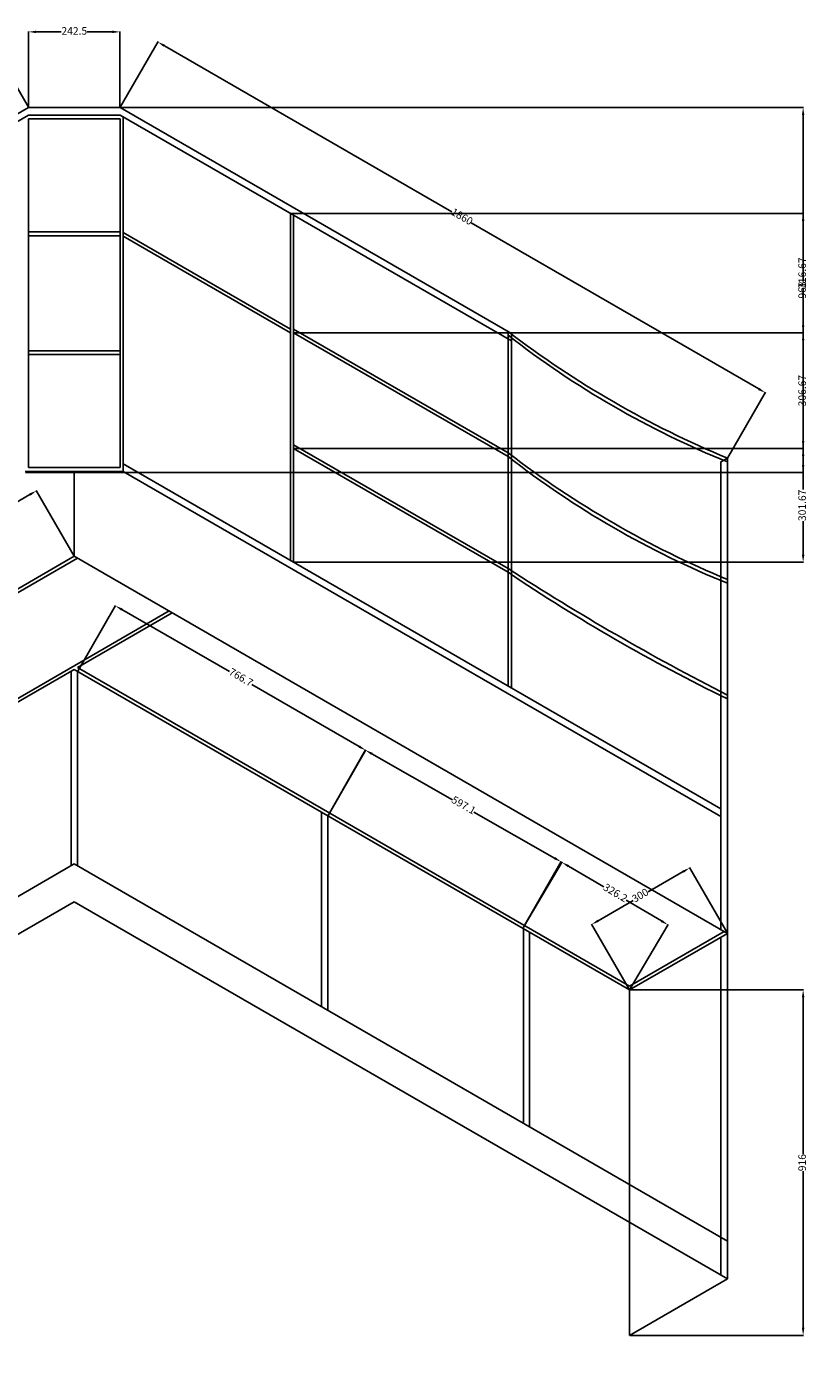
# Model space of a CAD drawing. Units: millimetres. Extents: x 78378 to 86415, y 148682 to 152721.
# Tile 18 of 18: x 84344 to 86415, y 149152 to 152721. Entities that reach past the tile are written whole.
import ezdxf

# ---------------------------------------------------------------- set-up
doc = ezdxf.new("R2010")
doc.units = ezdxf.units.MM
for name, color, linetype, lineweight in [('A-ANNO-DIMS', 2, 'Continuous', 18), ('A-ANNO-NPLT', 8, 'Continuous', 13), ('A-FURN', 4, 'Continuous', 25)]:
    doc.layers.add(name, color=color, linetype=linetype, lineweight=lineweight)
doc.styles.get("Standard").update_dxf_attribs({"font": 'arial.ttf'})
doc.dimstyles.new('ISO-25', dxfattribs={"dimtxt": 20, "dimasz": 20, "dimexe": 1.25, "dimexo": 0.625, "dimtad": 0, "dimdec": 1, "dimtxsty": 'Standard', "dimcen": 2.5, "dimadec": 0, "dimazin": 0, "dimtfac": 1, "dimtdec": 1, "dimtmove": 0, "dimatfit": 3, "dimfxl": 1, "dimarcsym": 0})

# ---------------------------------------------------------------- blocks, each defined once
blk = doc.blocks.new('*D35')
at = {"layer": 'A-ANNO-DIMS', "color": 0, "lineweight": -2, "transparency": 16777216}
for p, q in [((84347.7, 152508.2), (84247.2, 152682.4)), ((84230.5, 152671.3), (83252.4, 152106.6)), ((82221.3, 151511.3), (83199.4, 152076)), ((82303.9, 151328.2), (82203.4, 151502.4))]:
    blk.add_line(p, q, dxfattribs=at)
at = {"layer": 'A-ANNO-DIMS', "color": 0, "transparency": 16777216}
for points in [[(84228.8, 152674.2), (84232.2, 152668.4), (84247.8, 152681.3)], [(82219.6, 151514.2), (82223, 151508.4), (82204, 151501.3)]]:
    blk.add_solid(points, dxfattribs=at)
at = {"layer": 'Defpoints', "color": 0, "transparency": 16777216}
for p in [(84247.8, 152681.3), (84348.1, 152507.7), (82304.2, 151327.7)]:
    blk.add_point(p, dxfattribs=at)
at = {"layer": 'A-ANNO-DIMS', "color": 0, "transparency": 16777216, "insert": (83225.9, 152091.3), "char_height": 20, "attachment_point": 5, "rotation": 30}
blk.add_mtext('2360', dxfattribs=at)
blk = doc.blocks.new('*D36')
at = {"layer": 'A-ANNO-DIMS', "color": 0, "lineweight": -2, "transparency": 16777216}
for p, q in [((84590.9, 152508.2), (84691.4, 152682.4)), ((84708.1, 152671.3), (85470.6, 152231.1)), ((86284.3, 151761.3), (85521.8, 152201.6)), ((86201.7, 151578.2), (86302.2, 151752.4))]:
    blk.add_line(p, q, dxfattribs=at)
at = {"layer": 'A-ANNO-DIMS', "color": 0, "transparency": 16777216}
for points in [[(84709.8, 152674.2), (84706.5, 152668.4), (84690.8, 152681.3)], [(86286, 151764.2), (86282.6, 151758.4), (86301.6, 151751.3)]]:
    blk.add_solid(points, dxfattribs=at)
at = {"layer": 'Defpoints', "color": 0, "transparency": 16777216}
for p in [(84590.5, 152507.7), (86301.6, 151751.3), (86201.4, 151577.7)]:
    blk.add_point(p, dxfattribs=at)
at = {"layer": 'A-ANNO-DIMS', "color": 0, "transparency": 16777216, "insert": (85496.2, 152216.3), "char_height": 20, "attachment_point": 5, "rotation": 330}
blk.add_mtext('1860', dxfattribs=at)
blk = doc.blocks.new('*D37')
at = {"layer": 'A-ANNO-DIMS', "color": 0, "lineweight": -2, "transparency": 16777216}
for p, q in [((84348.1, 152508.3), (84348.1, 152709.4)), ((84590.5, 152508.3), (84590.5, 152709.4)), ((84368.1, 152708.2), (84434.7, 152708.2)), ((84570.5, 152708.2), (84503.9, 152708.2))]:
    blk.add_line(p, q, dxfattribs=at)
at = {"layer": 'A-ANNO-DIMS', "color": 0, "transparency": 16777216}
for points in [[(84368.1, 152711.5), (84368.1, 152704.9), (84348.1, 152708.2)], [(84570.5, 152711.5), (84570.5, 152704.9), (84590.5, 152708.2)]]:
    blk.add_solid(points, dxfattribs=at)
at = {"layer": 'Defpoints', "color": 0, "transparency": 16777216}
for p in [(84590.5, 152708.2), (84348.1, 152507.7), (84590.5, 152507.7)]:
    blk.add_point(p, dxfattribs=at)
at = {"layer": 'A-ANNO-DIMS', "color": 0, "transparency": 16777216, "insert": (84469.3, 152708.2), "char_height": 20, "attachment_point": 5}
blk.add_mtext('242.5', dxfattribs=at)
blk = doc.blocks.new('*D38')
at = {"layer": 'A-ANNO-DIMS', "color": 0, "lineweight": -2, "transparency": 16777216}
for p, q in [((84348.7, 152507.7), (86403.1, 152507.7)), ((86401.9, 152487.7), (86401.9, 152046.5)), ((86401.9, 151559.8), (86401.9, 152001)), ((84340, 151539.8), (86403.1, 151539.8))]:
    blk.add_line(p, q, dxfattribs=at)
at = {"layer": 'A-ANNO-DIMS', "color": 0, "transparency": 16777216}
for points in [[(86398.5, 152487.7), (86405.2, 152487.7), (86401.9, 152507.7)], [(86398.5, 151559.8), (86405.2, 151559.8), (86401.9, 151539.8)]]:
    blk.add_solid(points, dxfattribs=at)
at = {"layer": 'Defpoints', "color": 0, "transparency": 16777216}
for p in [(84348.1, 152507.7), (86401.9, 152507.7), (84339.4, 151539.8)]:
    blk.add_point(p, dxfattribs=at)
at = {"layer": 'A-ANNO-DIMS', "color": 0, "transparency": 16777216, "insert": (86401.9, 152023.7), "char_height": 20, "attachment_point": 5, "rotation": 90}
blk.add_mtext('968', dxfattribs=at)
blk = doc.blocks.new('*D41')
at = {"layer": 'A-ANNO-DIMS', "color": 0, "lineweight": -2, "transparency": 16777216}
for p, q in [((84351.7, 151481.3), (83937.7, 151242.3)), ((84469, 151318.2), (84368.4, 151492.4)), ((83452.3, 150962), (83866.3, 151201.1)), ((83534.9, 150778.9), (83434.4, 150953.1))]:
    blk.add_line(p, q, dxfattribs=at)
at = {"layer": 'A-ANNO-DIMS', "color": 0, "transparency": 16777216}
for points in [[(84350.1, 151484.2), (84353.4, 151478.4), (84369.1, 151491.3)], [(83450.6, 150964.9), (83454, 150959.2), (83435, 150952)]]:
    blk.add_solid(points, dxfattribs=at)
at = {"layer": 'Defpoints', "color": 0, "transparency": 16777216}
for p in [(84369.1, 151491.3), (84469.3, 151317.7), (83535.2, 150778.4)]:
    blk.add_point(p, dxfattribs=at)
at = {"layer": 'A-ANNO-DIMS', "color": 0, "transparency": 16777216, "insert": (83902, 151221.7), "char_height": 20, "attachment_point": 5, "rotation": 30}
blk.add_mtext('1078.6', dxfattribs=at)
blk = doc.blocks.new('*D46')
at = {"layer": 'A-ANNO-DIMS', "color": 0, "lineweight": -2, "transparency": 16777216}
for p, q in [((85942.2, 150167.7), (86403.1, 150167.7)), ((86401.9, 150147.7), (86401.9, 149732.4)), ((86401.9, 149271.7), (86401.9, 149687)), ((85942.2, 149251.7), (86403.1, 149251.7))]:
    blk.add_line(p, q, dxfattribs=at)
at = {"layer": 'A-ANNO-DIMS', "color": 0, "transparency": 16777216}
for points in [[(86398.5, 150147.7), (86405.2, 150147.7), (86401.9, 150167.7)], [(86398.5, 149271.7), (86405.2, 149271.7), (86401.9, 149251.7)]]:
    blk.add_solid(points, dxfattribs=at)
at = {"layer": 'Defpoints', "color": 0, "transparency": 16777216}
for p in [(85941.5, 150167.7), (86401.9, 150167.7), (85941.5, 149251.7)]:
    blk.add_point(p, dxfattribs=at)
at = {"layer": 'A-ANNO-DIMS', "color": 0, "transparency": 16777216, "insert": (86401.9, 149709.7), "char_height": 20, "attachment_point": 5, "rotation": 90}
blk.add_mtext('916', dxfattribs=at)
blk = doc.blocks.new('*D47')
at = {"layer": 'A-ANNO-DIMS', "color": 0, "lineweight": -2, "transparency": 16777216}
for p, q in [((84478.3, 151013.2), (84578.8, 151187.4)), ((84595.5, 151176.3), (84880.5, 151011.8)), ((85224.8, 150813), (84939.9, 150977.5)), ((85142.2, 150629.9), (85242.8, 150804.1))]:
    blk.add_line(p, q, dxfattribs=at)
at = {"layer": 'A-ANNO-DIMS', "color": 0, "transparency": 16777216}
for points in [[(84597.2, 151179.2), (84593.9, 151173.4), (84578.2, 151186.3)], [(85226.5, 150815.9), (85223.2, 150810.1), (85242.2, 150803)]]:
    blk.add_solid(points, dxfattribs=at)
at = {"layer": 'Defpoints', "color": 0, "transparency": 16777216}
for p in [(84478, 151012.7), (85242.2, 150803), (85141.9, 150629.4)]:
    blk.add_point(p, dxfattribs=at)
at = {"layer": 'A-ANNO-DIMS', "color": 0, "transparency": 16777216, "insert": (84910.2, 150994.7), "char_height": 20, "attachment_point": 5, "rotation": 330}
blk.add_mtext('766.7', dxfattribs=at)
blk = doc.blocks.new('*D48')
at = {"layer": 'A-ANNO-DIMS', "color": 0, "lineweight": -2, "transparency": 16777216}
for p, q in [((85142.2, 150629.9), (85241.9, 150804.6)), ((85258.7, 150793.6), (85472.4, 150671.6)), ((85742.5, 150517.4), (85528.8, 150639.4)), ((85660.8, 150333.9), (85760.5, 150508.6))]:
    blk.add_line(p, q, dxfattribs=at)
at = {"layer": 'A-ANNO-DIMS', "color": 0, "transparency": 16777216}
for points in [[(85260.3, 150796.5), (85257, 150790.7), (85241.3, 150803.5)], [(85744.2, 150520.3), (85740.9, 150514.5), (85759.9, 150507.5)]]:
    blk.add_solid(points, dxfattribs=at)
at = {"layer": 'Defpoints', "color": 0, "transparency": 16777216}
for p in [(85141.9, 150629.4), (85759.9, 150507.5), (85660.5, 150333.4)]:
    blk.add_point(p, dxfattribs=at)
at = {"layer": 'A-ANNO-DIMS', "color": 0, "transparency": 16777216, "insert": (85500.6, 150655.5), "char_height": 20, "attachment_point": 5, "rotation": 330.2843}
blk.add_mtext('597.1', dxfattribs=at)
blk = doc.blocks.new('*D49')
at = {"layer": 'A-ANNO-DIMS', "color": 0, "lineweight": -2, "transparency": 16777216}
for p, q in [((85660.8, 150333.9), (85763, 150507.2)), ((85779.6, 150495.9), (85873.3, 150440.7)), ((86026.1, 150350.6), (85932.4, 150405.9)), ((85941.9, 150168.2), (86044, 150341.5))]:
    blk.add_line(p, q, dxfattribs=at)
at = {"layer": 'A-ANNO-DIMS', "color": 0, "transparency": 16777216}
for points in [[(85781.3, 150498.8), (85777.9, 150493.1), (85762.3, 150506.1)], [(86027.8, 150353.4), (86024.5, 150347.7), (86043.4, 150340.4)]]:
    blk.add_solid(points, dxfattribs=at)
at = {"layer": 'Defpoints', "color": 0, "transparency": 16777216}
for p in [(85660.5, 150333.4), (86043.4, 150340.4), (85941.5, 150167.7)]:
    blk.add_point(p, dxfattribs=at)
at = {"layer": 'A-ANNO-DIMS', "color": 0, "transparency": 16777216, "insert": (85902.9, 150423.3), "char_height": 20, "attachment_point": 5, "rotation": 329.4797}
blk.add_mtext('326.2', dxfattribs=at)
blk = doc.blocks.new('*D50')
at = {"layer": 'A-ANNO-DIMS', "color": 0, "lineweight": -2, "transparency": 16777216}
for p, q in [((86083.8, 150481.3), (85990.8, 150427.7)), ((86201, 150318.2), (86100.5, 150492.4)), ((85858.6, 150351.3), (85951.6, 150405)), ((85941.2, 150168.2), (85840.7, 150342.4))]:
    blk.add_line(p, q, dxfattribs=at)
at = {"layer": 'A-ANNO-DIMS', "color": 0, "transparency": 16777216}
for points in [[(86082.1, 150484.2), (86085.5, 150478.4), (86101.1, 150491.3)], [(85857, 150354.2), (85860.3, 150348.4), (85841.3, 150341.3)]]:
    blk.add_solid(points, dxfattribs=at)
at = {"layer": 'Defpoints', "color": 0, "transparency": 16777216}
for p in [(86101.1, 150491.3), (86201.4, 150317.7), (85941.5, 150167.7)]:
    blk.add_point(p, dxfattribs=at)
at = {"layer": 'A-ANNO-DIMS', "color": 0, "transparency": 16777216, "insert": (85971.2, 150416.3), "char_height": 20, "attachment_point": 5, "rotation": 30}
blk.add_mtext('300', dxfattribs=at)
blk = doc.blocks.new('*D51')
at = {"layer": 'A-ANNO-DIMS', "color": 0, "lineweight": -2, "transparency": 16777216}
for p, q in [((85051.6, 151603.5), (86403.1, 151603.5)), ((86401.9, 151583.5), (86401.9, 151494.8)), ((86401.9, 151321.9), (86401.9, 151410.6)), ((85051.6, 151301.9), (86403.1, 151301.9))]:
    blk.add_line(p, q, dxfattribs=at)
at = {"layer": 'A-ANNO-DIMS', "color": 0, "transparency": 16777216}
for points in [[(86398.5, 151583.5), (86405.2, 151583.5), (86401.9, 151603.5)], [(86398.5, 151321.9), (86405.2, 151321.9), (86401.9, 151301.9)]]:
    blk.add_solid(points, dxfattribs=at)
at = {"layer": 'Defpoints', "color": 0, "transparency": 16777216}
for p in [(85051, 151603.5), (86401.9, 151603.5), (85051, 151301.9)]:
    blk.add_point(p, dxfattribs=at)
at = {"layer": 'A-ANNO-DIMS', "color": 0, "transparency": 16777216, "insert": (86401.9, 151452.7), "char_height": 20, "attachment_point": 5, "rotation": 90}
blk.add_mtext('301.67', dxfattribs=at)
blk = doc.blocks.new('*D52')
at = {"layer": 'A-ANNO-DIMS', "color": 0, "lineweight": -2, "transparency": 16777216}
for p, q in [((85051.6, 151910.2), (86403.1, 151910.2)), ((86401.9, 151890.2), (86401.9, 151799)), ((86401.9, 151623.5), (86401.9, 151714.7)), ((85051.6, 151603.5), (86403.1, 151603.5))]:
    blk.add_line(p, q, dxfattribs=at)
at = {"layer": 'A-ANNO-DIMS', "color": 0, "transparency": 16777216}
for points in [[(86398.5, 151890.2), (86405.2, 151890.2), (86401.9, 151910.2)], [(86398.5, 151623.5), (86405.2, 151623.5), (86401.9, 151603.5)]]:
    blk.add_solid(points, dxfattribs=at)
at = {"layer": 'Defpoints', "color": 0, "transparency": 16777216}
for p in [(85051, 151910.2), (86401.9, 151910.2), (85051, 151603.5)]:
    blk.add_point(p, dxfattribs=at)
at = {"layer": 'A-ANNO-DIMS', "color": 0, "transparency": 16777216, "insert": (86401.9, 151756.9), "char_height": 20, "attachment_point": 5, "rotation": 90}
blk.add_mtext('306.67', dxfattribs=at)
blk = doc.blocks.new('*D53')
at = {"layer": 'A-ANNO-DIMS', "color": 0, "lineweight": -2, "transparency": 16777216}
for p, q in [((85043, 152226.9), (86403.1, 152226.9)), ((86401.9, 152206.9), (86401.9, 152110.7)), ((86401.9, 151930.2), (86401.9, 152026.4)), ((85051.6, 151910.2), (86403.1, 151910.2))]:
    blk.add_line(p, q, dxfattribs=at)
at = {"layer": 'A-ANNO-DIMS', "color": 0, "transparency": 16777216}
for points in [[(86398.5, 152206.9), (86405.2, 152206.9), (86401.9, 152226.9)], [(86398.5, 151930.2), (86405.2, 151930.2), (86401.9, 151910.2)]]:
    blk.add_solid(points, dxfattribs=at)
at = {"layer": 'Defpoints', "color": 0, "transparency": 16777216}
for p in [(85042.3, 152226.9), (86401.9, 152226.9), (85051, 151910.2)]:
    blk.add_point(p, dxfattribs=at)
at = {"layer": 'A-ANNO-DIMS', "color": 0, "transparency": 16777216, "insert": (86401.9, 152068.5), "char_height": 20, "attachment_point": 5, "rotation": 90}
blk.add_mtext('316.67', dxfattribs=at)

msp = doc.modelspace()

# ---------------------------------------------------------------- linework, layer by layer
at = {"layer": 'A-ANNO-NPLT'}
for p in [(85046.6562, 152224.3613), (84348.0623, 152172.6946), (84590.5495, 152172.6946), (85050.9863, 151915.1946), (84348.0623, 151857.6946), (84590.5495, 151857.6946), (85050.9863, 151608.528), (85628.3366, 151581.8613), (85628.3366, 151275.1946)]:
    msp.add_point(p, dxfattribs=at)
at = {"layer": 'A-FURN'}
for p, q in [((82304.2424, 151327.6946), (84348.0623, 152507.6946)), ((84590.5495, 152507.6946), (84348.0623, 152507.6946)), ((84590.5495, 152507.6946), (85628.3366, 151908.528)), ((83953.1548, 152259.6946), (84348.0623, 152487.6946)), ((84348.0623, 152487.6946), (84590.5495, 152487.6946)), ((84348.0623, 152477.6946), (84348.0623, 151552.6946)), ((84348.0623, 152477.6946), (84590.5495, 152477.6946)), ((84590.5495, 152487.6946), (85628.3366, 151888.528)), ((84590.5495, 152477.6946), (84590.5495, 151552.6946)), ((84599.2097, 152482.6946), (84599.2097, 151542.6946)), ((85042.326, 152226.8613), (85042.326, 151306.8613)), ((85050.9863, 152221.8613), (85050.9863, 151301.8613)), ((84590.5495, 152177.6946), (84348.0623, 152177.6946)), ((85042.326, 151920.1946), (84599.2097, 152176.028)), ((84590.5495, 152167.6946), (84348.0623, 152167.6946)), ((85042.326, 151910.1946), (84599.2097, 152166.028)), ((85050.9863, 151920.1946), (85619.6763, 151591.8613)), ((85050.9863, 151910.1946), (85619.6763, 151581.8613)), ((85619.6763, 151913.528), (85619.6763, 150973.528)), ((85628.3366, 151908.528), (85628.3366, 150968.528)), ((84348.0623, 151862.6946), (84590.5495, 151862.6946)), ((84348.0623, 151852.6946), (84590.5495, 151852.6946)), ((85050.9863, 151613.528), (85619.6763, 151285.1946)), ((85050.9863, 151603.528), (85619.6763, 151275.1946)), ((86184.0362, 151567.6946), (86201.3567, 151577.6946)), ((86184.0362, 151567.6946), (86184.0362, 150327.6946)), ((86201.3567, 151577.6946), (86201.3567, 149401.6946)), ((84599.2097, 151542.6946), (84339.4021, 151542.6946)), ((84590.5495, 151552.6946), (84348.0623, 151552.6946)), ((84469.3059, 151542.6946), (84469.3059, 151317.6946)), ((84469.3059, 151542.6946), (84469.3059, 151317.6946)), ((84599.2097, 151562.6946), (86184.0362, 150647.6946)), ((84599.2097, 151542.6946), (86184.0362, 150627.6946)), ((84469.3059, 151317.6946), (83535.2323, 150778.407)), ((84469.3059, 151317.6946), (86201.3567, 150317.6946)), ((84477.9662, 151312.6946), (83535.2323, 150768.407)), ((84720.4533, 151172.6946), (83535.2323, 150488.407)), ((84477.9662, 151022.6946), (84729.1135, 151167.6946)), ((84469.3059, 151017.6946), (83535.2323, 150478.407)), ((84460.6456, 151012.6946), (84460.6456, 150496.6946)), ((84460.6456, 151012.6946), (84460.6456, 150496.6946)), ((84469.3059, 151017.6946), (85941.5491, 150167.6946)), ((84477.9662, 151022.6946), (85941.5491, 150177.6946)), ((84477.9662, 151012.6946), (84477.9662, 150496.6946)), ((84477.9662, 151012.6946), (84477.9662, 150496.6946)), ((85124.5985, 150639.3613), (85124.5985, 150123.3613)), ((85141.919, 150629.3613), (85141.919, 150113.3613)), ((83543.8926, 149967.407), (84469.3059, 150501.6946)), ((84469.3059, 150501.6946), (86201.3567, 149501.6946)), ((82304.2424, 149151.6946), (84469.3059, 150401.6946)), ((84469.3059, 150401.6946), (86201.3567, 149401.6946)), ((85660.5176, 150333.3692), (85660.5176, 149817.3692)), ((85675.968, 150321.028), (85675.968, 149805.028)), ((85941.5491, 150177.6946), (86192.6965, 150322.6946)), ((85941.5491, 150167.6946), (86201.3567, 150317.6946)), ((86184.0362, 150307.6946), (86184.0362, 149411.6946)), ((85941.5491, 149251.6946), (85941.5491, 150167.6946)), ((86201.3567, 149401.6946), (85941.5491, 149251.6946))]:
    msp.add_line(p, q, dxfattribs=at)
for centre, radius, start, end in [((87200.6508, 153980.1894), 2602.0318, 232.5843878, 247.4156122), ((87119.6642, 153829.9165), 2441.5029, 232.0937908, 247.9062092), ((87200.6508, 153658.5227), 2602.0318, 232.5843878, 247.4156122), ((87119.6642, 153508.2499), 2441.5029, 232.0937908, 247.9062092), ((89190.7083, 156798.8207), 6569.1184, 237.07034061, 242.92965939), ((88284.6881, 155219.4638), 4760.2045, 235.954411, 244.045589)]:
    msp.add_arc(centre, radius, start, end, dxfattribs=at)

# ---------------------------------------------------------------- dimensions: what is measured, and where the dimension line sits
at = {"layer": 'A-ANNO-DIMS'}
dim = msp.add_linear_dim(base=(84590.5495, 152708.1946), p1=(84348.0623, 152507.6946), p2=(84590.5495, 152507.6946), dimstyle='ISO-25', override={"dimdec": 1, "dimlfac": 1, "dimrnd": 0, "dimzin": 0, "dimdsep": 46, "dimlunit": 2}, dxfattribs=at)
dim.commit()
dim.dimension.update_dxf_attribs({"geometry": '*D37', "text_midpoint": (84469.3059, 152708.1946)})
for base, p1, p2, angle, override, picture, middle in [((84247.8123, 152681.3327), (82304.2424, 151327.6946), (84348.0623, 152507.6946), 30, {"dimdec": 0, "dimlfac": 1, "dimrnd": 0, "dimzin": 0, "dimdsep": 46, "dimlunit": 2}, '*D35', (83225.9024, 152091.3327)), ((86301.6067, 151751.3327), (84590.5495, 152507.6946), (86201.3567, 151577.6946), 330, {"dimdec": 0, "dimlfac": 1, "dimrnd": 0, "dimzin": 0, "dimdsep": 46, "dimlunit": 2}, '*D36', (85496.2031, 152216.3327)), ((86401.8567, 152507.6946), (84339.4021, 151539.7603), (84348.0623, 152507.6946), 90, {"dimdec": 0, "dimlfac": 1, "dimrnd": 0, "dimzin": 0, "dimdsep": 46, "dimlunit": 2}, '*D38', (86401.8567, 152023.7274)), ((86401.8567, 152226.8613), (85050.9863, 151910.1946), (85042.326, 152226.8613), 90, {"dimdec": 2, "dimlfac": 1, "dimrnd": 0, "dimzin": 0, "dimdsep": 46, "dimlunit": 2}, '*D53', (86401.8567, 152068.528)), ((86401.8567, 151910.1946), (85050.9863, 151603.528), (85050.9863, 151910.1946), 90, {"dimdec": 2, "dimlfac": 1, "dimrnd": 0, "dimzin": 0, "dimdsep": 46, "dimlunit": 2}, '*D52', (86401.8567, 151756.8613)), ((86401.8567, 151603.528), (85050.9863, 151301.8613), (85050.9863, 151603.528), 90, {"dimdec": 2, "dimlfac": 1, "dimrnd": 0, "dimzin": 0, "dimdsep": 46, "dimlunit": 2}, '*D51', (86401.8567, 151452.6946)), ((84369.0559, 151491.3327), (83535.2323, 150778.407), (84469.3059, 151317.6946), 30, {"dimdec": 1, "dimlfac": 1, "dimrnd": 0, "dimzin": 0, "dimdsep": 46, "dimlunit": 2}, '*D41', (83902.0191, 151221.6889)), ((85242.169, 150802.9994), (84477.9662, 151012.6946), (85141.919, 150629.3613), 330, {"dimdec": 1, "dimlfac": 1, "dimrnd": 0, "dimzin": 0, "dimdsep": 46, "dimlunit": 2}, '*D47', (84910.1926, 150994.6661)), ((85759.9048, 150507.5026), (85141.919, 150629.3613), (85660.5176, 150333.3692), 330.2842773, {"dimdec": 1, "dimlfac": 1, "dimrnd": 0, "dimzin": 0, "dimdsep": 46, "dimlunit": 2}, '*D48', (85500.6055, 150655.4986)), ((86043.3718, 150340.4152), (85660.5176, 150333.3692), (85941.5491, 150167.6946), 329.4796631, {"dimdec": 1, "dimlfac": 1, "dimrnd": 0, "dimzin": 0, "dimdsep": 46, "dimlunit": 2}, '*D49', (85902.8561, 150423.2525)), ((86101.1067, 150491.3327), (85941.5491, 150167.6946), (86201.3567, 150317.6946), 30, {"dimdec": 0, "dimlfac": 1, "dimrnd": 0, "dimzin": 0, "dimdsep": 46, "dimlunit": 2}, '*D50', (85971.2029, 150416.3327)), ((86401.8567, 150167.6946), (85941.5491, 149251.6946), (85941.5491, 150167.6946), 90, {"dimdec": 0, "dimlfac": 1, "dimrnd": 0, "dimzin": 0, "dimdsep": 46, "dimlunit": 2}, '*D46', (86401.8567, 149709.6946))]:
    dim = msp.add_linear_dim(base=base, p1=p1, p2=p2, angle=angle, dimstyle='ISO-25', override=override, dxfattribs=at)
    dim.commit()
    dim.dimension.update_dxf_attribs({"geometry": picture, "text_midpoint": middle})

doc.saveas('drawing.dxf')
